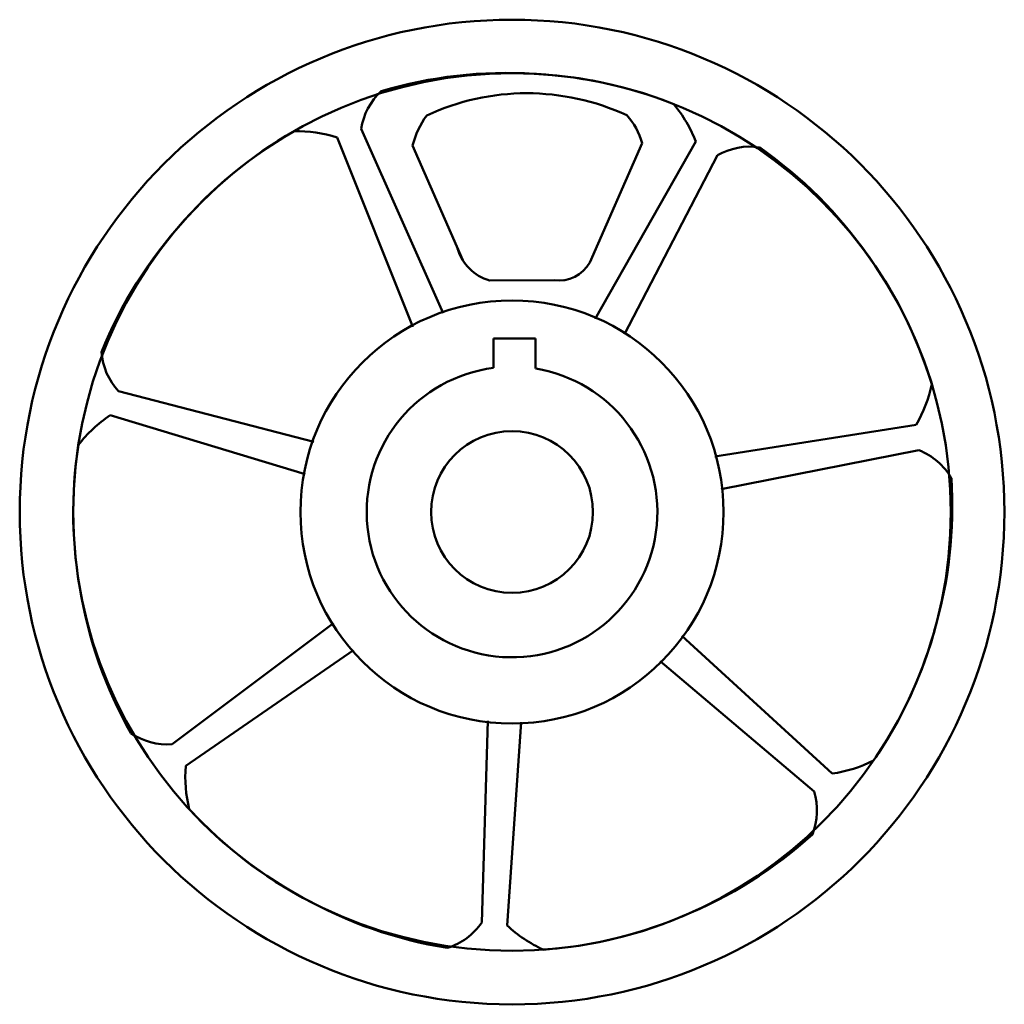
# Model space of a CAD drawing. Units: millimetres. Extents: x 1925 to 3748, y 659 to 2482.
import ezdxf

# ---------------------------------------------------------------- set-up
doc = ezdxf.new("R2010")
doc.units = ezdxf.units.MM
doc.layers.add('M-OUTL', color=7, linetype='Continuous', lineweight=50)

# ---------------------------------------------------------------- blocks, each defined once
blk = doc.blocks.new('*U1')
for p, q in [((-157.8, -217.2), (-309.9, 123.9)), ((123.2, -227.6), (309.9, 100.5))]:
    blk.add_line(p, q)
for centre, radius, start, end in [((-41.1, -584.8), 812.5, 86.3606, 106.5807), ((-30.5, -585.3), 812.5, 68.3487, 88.0498), ((-190.9, 105.8), 120.3, 132.9431, 171.342), ((70.3, 6.5), 257.4, 21.4207, 39.373)]:
    blk.add_arc(centre, radius, start, end)
blk = doc.blocks.new('*U2')
at = {"layer": 'M-OUTL', "color": 0, "linetype": 'ByBlock', "lineweight": -2, "transparency": 16777216}
blk.add_blockref('*U1', (2866.8, 2155.8), dxfattribs=at)
for p, rotation in [((2397.6, 1959.2), 51.42857142857145), ((3312.9, 1911.5), 308.5714285714287), ((2258.8, 1469.9), 102.8571428571429), ((3400.1, 1410.4), 257.1428571428572), ((2554.8, 1056.3), 154.2857142857143), ((3062.7, 1029.8), 205.7142857142857)]:
    blk.add_blockref('*U1', p, dxfattribs=dict(at, rotation=rotation))

msp = doc.modelspace()

# ---------------------------------------------------------------- linework, layer by layer
at = {"layer": 'M-OUTL'}
for p, q in [((2795.3, 2382.8), (2795.3, 2381.9)), ((2873.5, 2382), (2873.5, 2382)), ((2745, 2036.6), (2652.3, 2248.9)), ((3077.2, 2253.7), (2980.5, 2032.7)), ((2930.8, 1999.5), (2794.7, 1999.2)), ((2801.8, 1891.7), (2801.8, 1837.3)), ((2801.8, 1891.7), (2880, 1891.7)), ((2880, 1891.7), (2880, 1835.9))]:
    msp.add_line(p, q, dxfattribs=at)
for radius in [911.7, 812.5, 391.8]:
    msp.add_circle((2836.3, 1570.4), radius, dxfattribs=at)
at = {"layer": 'M-OUTL', "extrusion": (0, 0, -1)}
msp.add_circle((-2836.3, 1570.4), 149.9, dxfattribs=at)
at = {"layer": 'M-OUTL'}
for centre, radius, start, end in [((2863.7, 1906.4), 439.5, 65.1082, 114.9387), ((2805.8, 2211.4), 158.1, 143.7289, 166.2647), ((2959, 2221.7), 122.4, 15.1313, 42.9059), ((2817.6, 2081.4), 85.3, 195.5619, 254.4451), ((2922.6, 2065.5), 66.5, 263.1164, 330.4116), ((2836.3, 1570.4), 269.1, 97.3472, 80.6329)]:
    msp.add_arc(centre, radius, start, end, dxfattribs=at)

# ---------------------------------------------------------------- block references
msp.add_blockref('*U2', (0, 0), dxfattribs=at)

doc.saveas('drawing.dxf')
